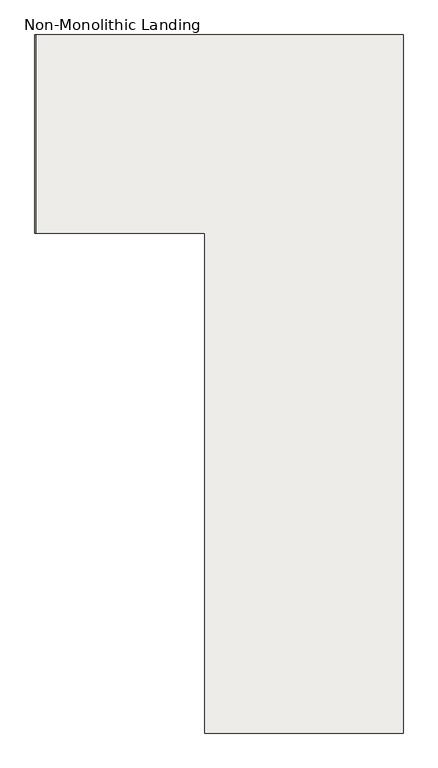
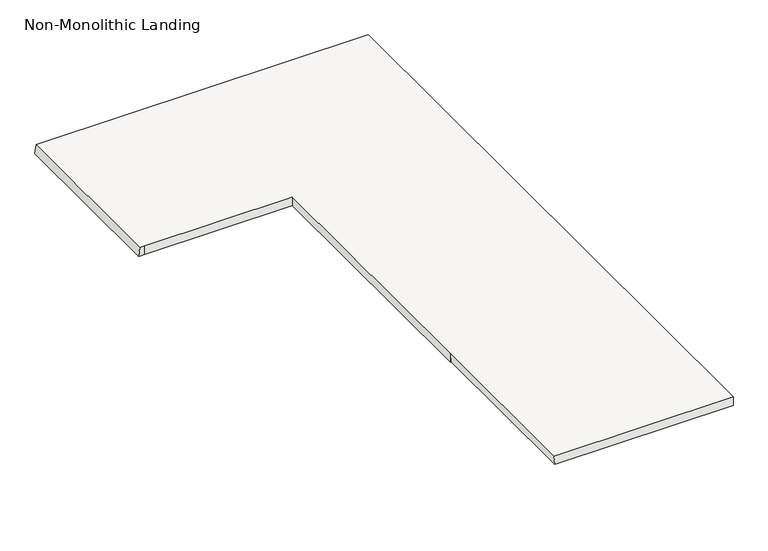
"""IFC4 building model written with IfcOpenShell, lengths in millimetres: slab geometry, Non-Monolithic Landing."""

from ifc_helpers import new_model, si_unit, origin, place, context, project, spatial, faceted_brep, source, transform, mapped, element, save


def non_monolithic_landing_a96adf93(model_context):
    return source(origin(), model_context, "Body", "Brep", [
        faceted_brep([(12350.7864069, -11.8843256, 1075.7647059), (12343.8146221, -11.8843256, 1025.7647059), (12343.8146221, -1011.9101069, 1025.7647059), (12350.7864069, -1011.9101069, 1075.7647059), (13200.7864069, -3533.7536983, 1075.7647059), (14200.8121881, -3533.7536983, 1075.7647059), (14200.8121881, -11.8843256, 1075.7647059), (12375.7864069, -11.8843256, 1075.7647059), (12375.7864069, -1011.9101069, 1075.7647059), (13200.7864069, -1011.9101069, 1075.7647059), (13200.7864069, -2533.727917, 1075.7647059), (14200.8121881, -11.8843256, 1025.7647059), (14200.8121881, -3533.7536983, 1025.7647059), (13207.7581917, -3533.7536983, 1025.7647059), (13207.7581917, -2533.727917, 1025.7647059), (13200.7864069, -2533.727917, 1025.7647059), (13200.7864069, -1011.9101069, 1025.7647059), (12375.7864069, -1011.9101069, 1025.7647059), (12375.7864069, -11.8843256, 1025.7647059)], [[[0, 1, 2, 3]], [[4, 5, 6, 7, 0, 3, 8, 9, 10]], [[11, 12, 13, 14, 15, 16, 17, 2, 1, 18]], [[5, 4, 13, 12]], [[6, 5, 12, 11]], [[7, 6, 11, 18]], [[0, 7, 18, 1]], [[8, 3, 2, 17]], [[9, 8, 17, 16]], [[10, 9, 16, 15]], [[14, 10, 15]], [[10, 14, 13, 4]]]),
    ])


if __name__ == "__main__":
    model = new_model("IFC4")
    model_context = context("Model", 3, world=origin())
    ifc_project = project(units=[si_unit("LENGTHUNIT", "METRE", prefix="MILLI")], contexts=[model_context])
    site = spatial("IfcSite", under=ifc_project)
    building = spatial("IfcBuilding", under=site)
    placement = place(None, origin())
    non_monolithic_landing_shape = non_monolithic_landing_a96adf93(model_context)
    element("IfcSlab", 1, ObjectType="Non-Monolithic Landing", at=placement, inside=building, context=model_context, shape_type="MappedRepresentation", body=[
        mapped(non_monolithic_landing_shape, transform((0.0, 0.0, 0.0), x_axis=(1.0, 0.0, 0.0), y_axis=(0.0, 1.0, 0.0), z_axis=(0.0, 0.0, 1.0))),
    ])
    save(model, "model.ifc")
